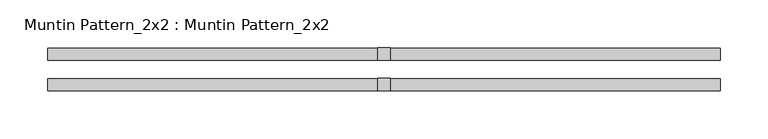
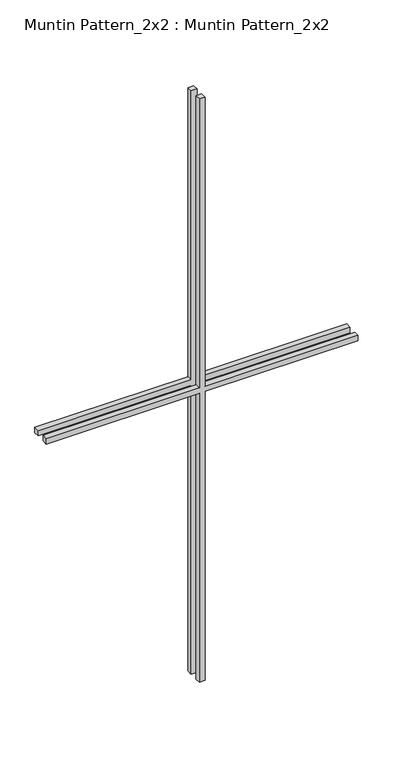
"""IFC4 building model written with IfcOpenShell, lengths in millimetres: proxy geometry, Muntin Pattern_2x2 : Muntin Pattern_2x2."""

from ifc_helpers import new_model, si_unit, frame, origin, place, context, project, spatial, polyline, outline, extrude, source, transform, mapped, element, save


def muntin_pattern_2x2_muntin_pattern_2x2_d8607f27(model_context):
    return source(origin(), model_context, "Body", "SweptSolid", [
        extrude(outline(polyline([(698.5, -6.35), (698.5, -350.2391737), (685.8, -350.2391737), (685.8, -6.35), (0.0, -6.35), (0.0, 6.35), (685.8, 6.35), (685.8, 350.2391737), (698.5, 350.2391737), (698.5, 6.35), (1384.3, 6.35), (1384.3, -6.35), (698.5, -6.35)])), frame((0.0, 9.525, 0.0), z_axis=(0.0, 1.0, 0.0), x_axis=(0.0, 0.0, 1.0)), (0.0, 0.0, 1.0), 12.7),
        extrude(outline(polyline([(698.5, -6.35), (698.5, -350.2391737), (685.8, -350.2391737), (685.8, -6.35), (0.0, -6.35), (0.0, 6.35), (685.8, 6.35), (685.8, 350.2391737), (698.5, 350.2391737), (698.5, 6.35), (1384.3, 6.35), (1384.3, -6.35), (698.5, -6.35)])), frame((0.0, -22.225, 0.0), z_axis=(0.0, 1.0, 0.0), x_axis=(0.0, 0.0, 1.0)), (0.0, 0.0, 1.0), 12.7),
    ])


if __name__ == "__main__":
    model = new_model("IFC4")
    model_context = context("Model", 3, world=origin())
    ifc_project = project(units=[si_unit("LENGTHUNIT", "METRE", prefix="MILLI")], contexts=[model_context])
    site = spatial("IfcSite", under=ifc_project)
    building = spatial("IfcBuilding", under=site)
    placement = place(None, origin())
    muntin_pattern_2x2_muntin_pattern_2x2_shape = muntin_pattern_2x2_muntin_pattern_2x2_d8607f27(model_context)
    element("IfcBuildingElementProxy", 1, Name="Muntin Pattern_2x2 : Muntin Pattern_2x2", ObjectType="Muntin Pattern_2x2 : Muntin Pattern_2x2", at=placement, inside=building, context=model_context, shape_type="MappedRepresentation", body=[
        mapped(muntin_pattern_2x2_muntin_pattern_2x2_shape, transform((0.0, 0.0, 0.0), x_axis=(1.0, 0.0, 0.0), y_axis=(0.0, 1.0, 0.0), z_axis=(0.0, 0.0, 1.0))),
    ])
    save(model, "model.ifc")

# Revit data of these elements
# Type "Muntin Pattern_2x2 : Muntin Pattern_2x2"
#   Width [instance default] = 4' - 0"
#   Thickness = 0' - 0 1/2"
#   Height [instance default] = 4' - 0"
#   Distance = 0' - 0 3/4"
#   Interior Material [instance default] = none
#   Exterior Material [instance default] = none
#   Default Elevation = 0
# Element 1 (IfcBuildingElementProxy, "Muntin Pattern_2x2 : Muntin Pattern_2x2")
#   Width = 2' - 3.57789"
#   Height = 4' - 6 1/2"
#   Interior Material = Wood - Stained
#   Exterior Material = Clad - White
#   Materials on its faces: "Clad - White", "Wood - Stained"
# Materials
#   "Clad - White": class "Wood", colour RGB 242 242 238, transparency 0, Cost = 0
#   "Wood - Stained": class "Wood", colour RGB 224 178 126, transparency 0, Cost = 0
